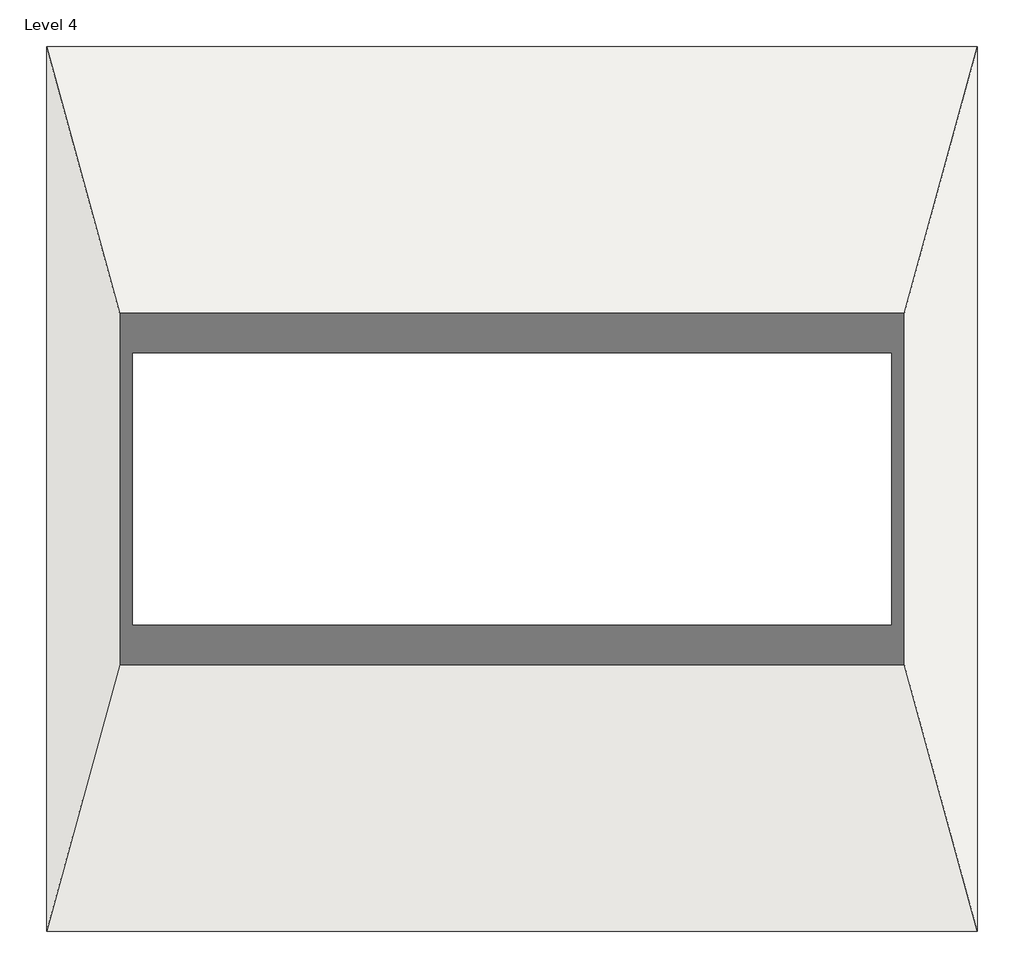
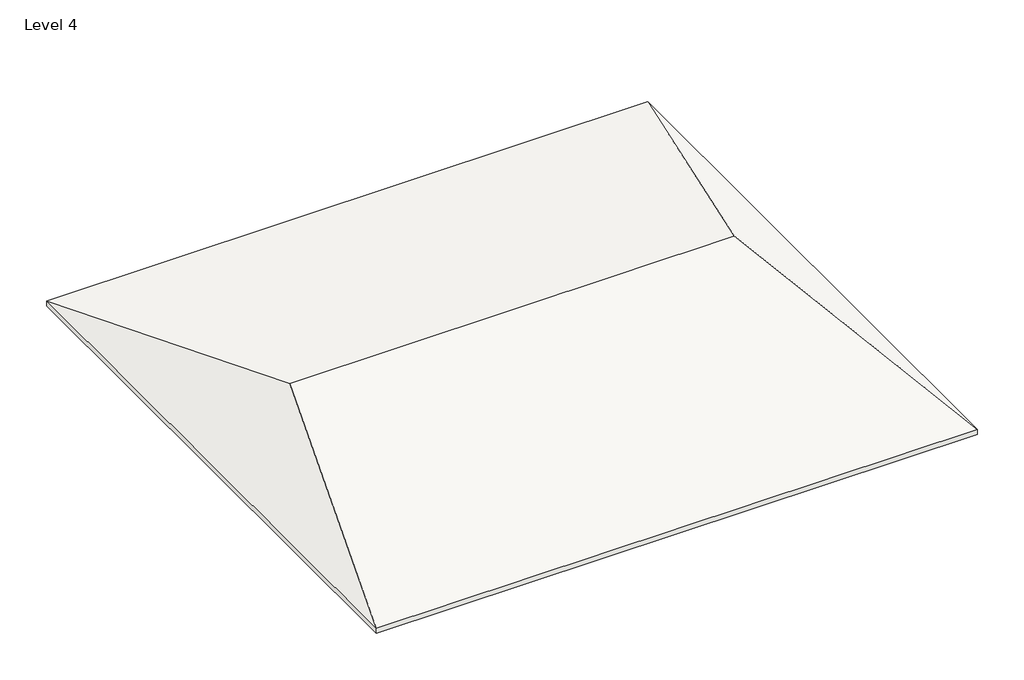
# One storey: 1 roof.
"""IFC4 building model written with IfcOpenShell, lengths in millimetres."""

from ifc_helpers import new_model, si_unit, origin, place, context, project, spatial, faceted_brep, element, save

model = new_model("IFC4")

# Units and contexts
model_context = context("Model", 3, world=origin())
ifc_project = project(units=[si_unit("LENGTHUNIT", "METRE", prefix="MILLI")], contexts=[model_context])

# Site, building, storey
site = spatial("IfcSite", under=ifc_project)
building = spatial("IfcBuilding", under=site)
storey = spatial("IfcBuildingStorey", under=building, Name="Level 4", Elevation=6858.0)

# Roof
placement = place(None, origin())
element("IfcRoof", 1, ObjectType="6\" roof", at=placement, inside=storey, context=model_context, shape_type="Brep", body=[
    faceted_brep([(8021.1071817, 9396.8050084, 6858.0), (5712.854933, 958.3410124, 8589.1891865), (-7332.1047861, 958.3410124, 8589.1891865), (-9640.3570347, 9396.8050084, 6858.0), (-9640.3570347, -7480.1229837, 6858.0), (8021.1071817, -7480.1229837, 6858.0), (8067.6750735, 9396.8050084, 7013.5740811), (-9686.9249265, 9396.8050084, 7013.5740811), (-7378.6726779, 958.3410124, 8744.7632676), (5759.4228249, 958.3410124, 8744.7632676), (-9686.9249265, -7480.1229837, 7013.5740811), (8067.6750735, -7480.1229837, 7013.5740811), (-9686.9249265, 9396.8050084, 6858.0), (8067.6750735, 9396.8050084, 6858.0), (-9686.9249265, -7480.1229837, 6858.0), (8067.6750735, -7480.1229837, 6858.0)], [[[0, 1, 2, 3]], [[3, 2, 4]], [[4, 2, 1, 5]], [[1, 0, 5]], [[6, 7, 8, 9]], [[7, 10, 8]], [[10, 11, 9, 8]], [[6, 9, 11]], [[12, 7, 6, 13, 0, 3]], [[14, 10, 7, 12]], [[15, 11, 10, 14, 4, 5]], [[13, 6, 11, 15]], [[13, 15, 5, 0]], [[4, 14, 12, 3]]]),
])

save(model, "model.ifc")

# Revit data of these elements
# Type "6\" roof"
#   Assembly Code = "B1020"
#   Layers, outside or top first: 0' - 6" "roof" (function 1)
# Element 1 (IfcRoof, "6\" roof")
#   built-in parameter 1001705 = 28.6902 (stored number, unit not read)
#   built-in parameter 1001710 = 33615
#   Phase Created = New Construction
#   Materials on its faces: "roof"
# Materials
#   "roof": class "Generic", colour RGB 120 120 120, transparency 0, Cost = 0
